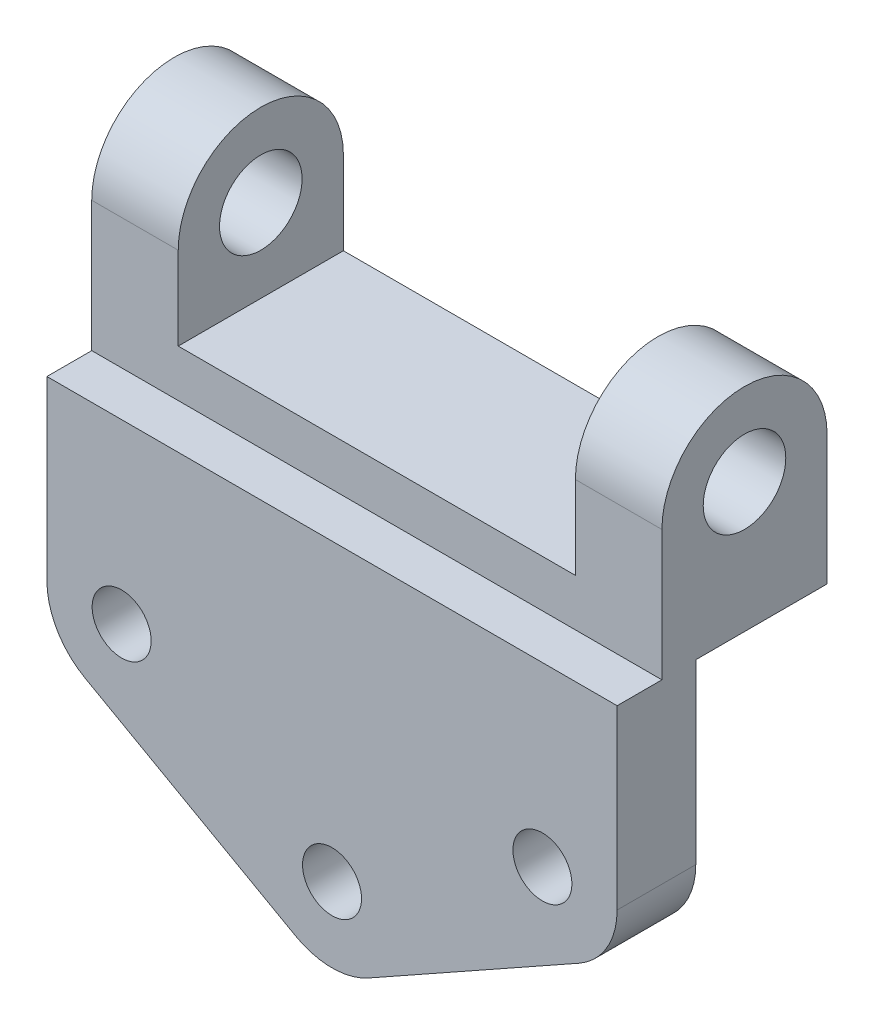
ISO-10303-21;
HEADER;
FILE_DESCRIPTION(('STEP AP214'),'2;1');
FILE_NAME('part.step','',(''),(''),'','','');
FILE_SCHEMA(('AUTOMOTIVE_DESIGN { 1 0 10303 214 1 1 1 1 }'));
ENDSEC;
DATA;
#1=APPLICATION_CONTEXT('core data for automotive mechanical design processes');
#2=APPLICATION_PROTOCOL_DEFINITION('international standard','automotive_design',2000,#1);
#3=PRODUCT_CONTEXT('',#1,'mechanical');
#4=PRODUCT('Part','Part','',(#3));
#5=PRODUCT_RELATED_PRODUCT_CATEGORY('part','',(#4));
#6=PRODUCT_DEFINITION_FORMATION('','',#4);
#7=PRODUCT_DEFINITION_CONTEXT('part definition',#1,'design');
#8=PRODUCT_DEFINITION('design','',#6,#7);
#9=PRODUCT_DEFINITION_SHAPE('','',#8);
#10=(LENGTH_UNIT() NAMED_UNIT(*) SI_UNIT(.MILLI.,.METRE.));
#11=(NAMED_UNIT(*) PLANE_ANGLE_UNIT() SI_UNIT($,.RADIAN.));
#12=(NAMED_UNIT(*) SI_UNIT($,.STERADIAN.) SOLID_ANGLE_UNIT());
#13=UNCERTAINTY_MEASURE_WITH_UNIT(LENGTH_MEASURE(1.E-05),#10,'distance_accuracy_value','');
#14=(GEOMETRIC_REPRESENTATION_CONTEXT(3) GLOBAL_UNCERTAINTY_ASSIGNED_CONTEXT((#13)) GLOBAL_UNIT_ASSIGNED_CONTEXT((#10,
#11,#12)) REPRESENTATION_CONTEXT('',''));
#15=CARTESIAN_POINT('',(0.,0.,0.));
#16=DIRECTION('',(0.,0.,1.));
#17=DIRECTION('',(1.,0.,0.));
#18=AXIS2_PLACEMENT_3D('',#15,#16,#17);
#19=CARTESIAN_POINT('',(72.5,33.,-12.3921818654785));
#20=DIRECTION('',(1.,0.,0.));
#21=DIRECTION('',(0.,0.,-1.));
#22=AXIS2_PLACEMENT_3D('',#19,#20,#21);
#23=PLANE('',#22);
#24=CARTESIAN_POINT('',(72.5,33.,-12.3921818654785));
#25=DIRECTION('',(1.,0.,0.));
#26=DIRECTION('',(0.,0.,-1.));
#27=AXIS2_PLACEMENT_3D('',#24,#25,#26);
#28=CIRCLE('',#27,10.5);
#29=CARTESIAN_POINT('',(72.5,33.,-22.8921818654785));
#30=VERTEX_POINT('',#29);
#31=EDGE_CURVE('E272',#30,#30,#28,.T.);
#32=ORIENTED_EDGE('',*,*,#31,.F.);
#33=EDGE_LOOP('',(#32));
#34=FACE_BOUND('',#33,.T.);
#35=DIRECTION('',(0.,-1.,0.));
#36=VECTOR('',#35,1.);
#37=CARTESIAN_POINT('',(72.5,-0.114515685512906,20.));
#38=LINE('',#37,#36);
#39=CARTESIAN_POINT('',(72.5,-0.114515685512906,20.));
#40=VERTEX_POINT('',#39);
#41=CARTESIAN_POINT('',(72.5,-45.1145156855129,20.));
#42=VERTEX_POINT('',#41);
#43=EDGE_CURVE('E288',#40,#42,#38,.T.);
#44=ORIENTED_EDGE('',*,*,#43,.T.);
#45=DIRECTION('',(0.,0.,1.));
#46=VECTOR('',#45,1.);
#47=CARTESIAN_POINT('',(72.5,-45.1145156855129,-125.));
#48=LINE('',#47,#46);
#49=CARTESIAN_POINT('',(72.5,-45.1145156855129,0.));
#50=VERTEX_POINT('',#49);
#51=EDGE_CURVE('E243',#50,#42,#48,.T.);
#52=ORIENTED_EDGE('',*,*,#51,.F.);
#53=DIRECTION('',(0.,1.,0.));
#54=VECTOR('',#53,1.);
#55=CARTESIAN_POINT('',(72.5,-75.1145156855129,0.));
#56=LINE('',#55,#54);
#57=CARTESIAN_POINT('',(72.5,0.,0.));
#58=VERTEX_POINT('',#57);
#59=EDGE_CURVE('E292',#50,#58,#56,.T.);
#60=ORIENTED_EDGE('',*,*,#59,.T.);
#61=DIRECTION('',(0.,0.,-1.));
#62=VECTOR('',#61,1.);
#63=CARTESIAN_POINT('',(72.5,0.,0.));
#64=LINE('',#63,#62);
#65=CARTESIAN_POINT('',(72.5,0.,-33.3921818654785));
#66=VERTEX_POINT('',#65);
#67=EDGE_CURVE('E291',#58,#66,#64,.T.);
#68=ORIENTED_EDGE('',*,*,#67,.T.);
#69=DIRECTION('',(0.,1.,0.));
#70=VECTOR('',#69,1.);
#71=CARTESIAN_POINT('',(72.5,0.,-33.3921818654785));
#72=LINE('',#71,#70);
#73=CARTESIAN_POINT('',(72.5,33.,-33.3921818654785));
#74=VERTEX_POINT('',#73);
#75=EDGE_CURVE('E293',#66,#74,#72,.T.);
#76=ORIENTED_EDGE('',*,*,#75,.T.);
#77=CARTESIAN_POINT('',(72.5,33.,-12.3921818654785));
#78=DIRECTION('',(1.,0.,0.));
#79=DIRECTION('',(0.,0.,-1.));
#80=AXIS2_PLACEMENT_3D('',#77,#78,#79);
#81=CIRCLE('',#80,21.);
#82=CARTESIAN_POINT('',(72.5,33.,8.60781813452149));
#83=VERTEX_POINT('',#82);
#84=EDGE_CURVE('E278',#74,#83,#81,.T.);
#85=ORIENTED_EDGE('',*,*,#84,.T.);
#86=DIRECTION('',(0.,-1.,0.));
#87=VECTOR('',#86,1.);
#88=CARTESIAN_POINT('',(72.5,33.,8.60781813452149));
#89=LINE('',#88,#87);
#90=CARTESIAN_POINT('',(72.5,-0.114515685512906,8.60781813452149));
#91=VERTEX_POINT('',#90);
#92=EDGE_CURVE('E282',#83,#91,#89,.T.);
#93=ORIENTED_EDGE('',*,*,#92,.T.);
#94=DIRECTION('',(0.,0.,1.));
#95=VECTOR('',#94,1.);
#96=CARTESIAN_POINT('',(72.5,-0.114515685512906,8.60781813452149));
#97=LINE('',#96,#95);
#98=EDGE_CURVE('E286',#91,#40,#97,.T.);
#99=ORIENTED_EDGE('',*,*,#98,.T.);
#100=EDGE_LOOP('',(#44,#52,#60,#68,#76,#85,#93,#99));
#101=FACE_BOUND('',#100,.T.);
#102=ADVANCED_FACE('F82',(#34,#101),#23,.T.);
#103=CARTESIAN_POINT('',(72.5,33.,-12.3921818654785));
#104=DIRECTION('',(-1.,0.,0.));
#105=DIRECTION('',(0.,0.,1.));
#106=AXIS2_PLACEMENT_3D('',#103,#104,#105);
#107=CYLINDRICAL_SURFACE('',#106,21.);
#108=CARTESIAN_POINT('',(50.5,33.,-12.3921818654785));
#109=DIRECTION('',(-1.,0.,0.));
#110=DIRECTION('',(0.,0.,1.));
#111=AXIS2_PLACEMENT_3D('',#108,#109,#110);
#112=CIRCLE('',#111,21.);
#113=CARTESIAN_POINT('',(50.5,33.,8.60781813452149));
#114=VERTEX_POINT('',#113);
#115=CARTESIAN_POINT('',(50.5,33.,-33.3921818654785));
#116=VERTEX_POINT('',#115);
#117=EDGE_CURVE('E264',#114,#116,#112,.T.);
#118=ORIENTED_EDGE('',*,*,#117,.F.);
#119=DIRECTION('',(-1.,0.,0.));
#120=VECTOR('',#119,1.);
#121=CARTESIAN_POINT('',(72.5,33.,8.60781813452149));
#122=LINE('',#121,#120);
#123=EDGE_CURVE('E327',#83,#114,#122,.T.);
#124=ORIENTED_EDGE('',*,*,#123,.F.);
#125=ORIENTED_EDGE('',*,*,#84,.F.);
#126=DIRECTION('',(-1.,0.,0.));
#127=VECTOR('',#126,1.);
#128=CARTESIAN_POINT('',(72.5,33.,-33.3921818654785));
#129=LINE('',#128,#127);
#130=EDGE_CURVE('E315',#74,#116,#129,.T.);
#131=ORIENTED_EDGE('',*,*,#130,.T.);
#132=EDGE_LOOP('',(#118,#124,#125,#131));
#133=FACE_BOUND('',#132,.T.);
#134=ADVANCED_FACE('F387',(#133),#107,.T.);
#135=CARTESIAN_POINT('',(72.5,33.,8.60781813452149));
#136=DIRECTION('',(0.,0.,-1.));
#137=DIRECTION('',(-1.,0.,0.));
#138=AXIS2_PLACEMENT_3D('',#135,#136,#137);
#139=PLANE('',#138);
#140=DIRECTION('',(0.,1.,0.));
#141=VECTOR('',#140,1.);
#142=CARTESIAN_POINT('',(50.5,33.,8.60781813452149));
#143=LINE('',#142,#141);
#144=CARTESIAN_POINT('',(50.5,11.8854843144871,8.60781813452149));
#145=VERTEX_POINT('',#144);
#146=EDGE_CURVE('E270',#145,#114,#143,.T.);
#147=ORIENTED_EDGE('',*,*,#146,.F.);
#148=DIRECTION('',(-1.,0.,0.));
#149=VECTOR('',#148,1.);
#150=CARTESIAN_POINT('',(72.5,11.8854843144871,8.60781813452149));
#151=LINE('',#150,#149);
#152=CARTESIAN_POINT('',(-50.5,11.8854843144871,8.60781813452149));
#153=VERTEX_POINT('',#152);
#154=EDGE_CURVE('E267',#145,#153,#151,.T.);
#155=ORIENTED_EDGE('',*,*,#154,.T.);
#156=DIRECTION('',(0.,1.,0.));
#157=VECTOR('',#156,1.);
#158=CARTESIAN_POINT('',(-50.5,33.,8.60781813452149));
#159=LINE('',#158,#157);
#160=CARTESIAN_POINT('',(-50.5,33.,8.60781813452149));
#161=VERTEX_POINT('',#160);
#162=EDGE_CURVE('E259',#153,#161,#159,.T.);
#163=ORIENTED_EDGE('',*,*,#162,.T.);
#164=CARTESIAN_POINT('',(-72.5,33.,8.60781813452149));
#165=VERTEX_POINT('',#164);
#166=EDGE_CURVE('E330',#161,#165,#122,.T.);
#167=ORIENTED_EDGE('',*,*,#166,.T.);
#168=DIRECTION('',(0.,-1.,0.));
#169=VECTOR('',#168,1.);
#170=CARTESIAN_POINT('',(-72.5,33.,8.60781813452149));
#171=LINE('',#170,#169);
#172=CARTESIAN_POINT('',(-72.5,-0.114515685512906,8.60781813452149));
#173=VERTEX_POINT('',#172);
#174=EDGE_CURVE('E296',#165,#173,#171,.T.);
#175=ORIENTED_EDGE('',*,*,#174,.T.);
#176=DIRECTION('',(-1.,0.,0.));
#177=VECTOR('',#176,1.);
#178=CARTESIAN_POINT('',(72.5,-0.114515685512906,8.60781813452149));
#179=LINE('',#178,#177);
#180=EDGE_CURVE('E322',#91,#173,#179,.T.);
#181=ORIENTED_EDGE('',*,*,#180,.F.);
#182=ORIENTED_EDGE('',*,*,#92,.F.);
#183=ORIENTED_EDGE('',*,*,#123,.T.);
#184=EDGE_LOOP('',(#147,#155,#163,#167,#175,#181,#182,#183));
#185=FACE_BOUND('',#184,.T.);
#186=ADVANCED_FACE('F386',(#185),#139,.F.);
#187=CARTESIAN_POINT('',(72.5,-0.114515685512906,20.));
#188=DIRECTION('',(0.,0.,-1.));
#189=DIRECTION('',(0.,1.,0.));
#190=AXIS2_PLACEMENT_3D('',#187,#188,#189);
#191=PLANE('',#190);
#192=DIRECTION('',(0.872227864306251,-0.489099736994159,0.));
#193=VECTOR('',#192,1.);
#194=CARTESIAN_POINT('',(-41.3372295567459,-73.718059376197,20.));
#195=LINE('',#194,#193);
#196=CARTESIAN_POINT('',(-62.792895002889,-61.6868451073317,20.));
#197=VERTEX_POINT('',#196);
#198=CARTESIAN_POINT('',(-9.29289500288903,-91.6868451073317,20.));
#199=VERTEX_POINT('',#198);
#200=EDGE_CURVE('E197',#197,#199,#195,.T.);
#201=ORIENTED_EDGE('',*,*,#200,.T.);
#202=CARTESIAN_POINT('',(0.,-75.1145156855129,20.));
#203=DIRECTION('',(0.,0.,1.));
#204=DIRECTION('',(1.,0.,0.));
#205=AXIS2_PLACEMENT_3D('',#202,#203,#204);
#206=CIRCLE('',#205,19.);
#207=CARTESIAN_POINT('',(9.29289500288903,-91.6868451073317,20.));
#208=VERTEX_POINT('',#207);
#209=EDGE_CURVE('E201',#199,#208,#206,.T.);
#210=ORIENTED_EDGE('',*,*,#209,.T.);
#211=DIRECTION('',(-0.872227864306251,-0.489099736994159,0.));
#212=VECTOR('',#211,1.);
#213=CARTESIAN_POINT('',(41.3372295567459,-73.718059376197,20.));
#214=LINE('',#213,#212);
#215=CARTESIAN_POINT('',(62.792895002889,-61.6868451073317,20.));
#216=VERTEX_POINT('',#215);
#217=EDGE_CURVE('E242',#216,#208,#214,.T.);
#218=ORIENTED_EDGE('',*,*,#217,.F.);
#219=CARTESIAN_POINT('',(53.5,-45.1145156855129,20.));
#220=DIRECTION('',(0.,0.,1.));
#221=DIRECTION('',(1.,0.,0.));
#222=AXIS2_PLACEMENT_3D('',#219,#220,#221);
#223=CIRCLE('',#222,19.);
#224=EDGE_CURVE('E246',#42,#216,#223,.F.);
#225=ORIENTED_EDGE('',*,*,#224,.F.);
#226=ORIENTED_EDGE('',*,*,#43,.F.);
#227=DIRECTION('',(-1.,0.,0.));
#228=VECTOR('',#227,1.);
#229=CARTESIAN_POINT('',(72.5,-0.114515685512906,20.));
#230=LINE('',#229,#228);
#231=CARTESIAN_POINT('',(-72.5,-0.114515685512906,20.));
#232=VERTEX_POINT('',#231);
#233=EDGE_CURVE('E321',#40,#232,#230,.T.);
#234=ORIENTED_EDGE('',*,*,#233,.T.);
#235=DIRECTION('',(0.,-1.,0.));
#236=VECTOR('',#235,1.);
#237=CARTESIAN_POINT('',(-72.5,-0.114515685512906,20.));
#238=LINE('',#237,#236);
#239=CARTESIAN_POINT('',(-72.5,-45.1145156855129,20.));
#240=VERTEX_POINT('',#239);
#241=EDGE_CURVE('E302',#232,#240,#238,.T.);
#242=ORIENTED_EDGE('',*,*,#241,.T.);
#243=CARTESIAN_POINT('',(-53.5,-45.1145156855129,20.));
#244=DIRECTION('',(0.,0.,1.));
#245=DIRECTION('',(1.,0.,0.));
#246=AXIS2_PLACEMENT_3D('',#243,#244,#245);
#247=CIRCLE('',#246,19.);
#248=EDGE_CURVE('E202',#240,#197,#247,.T.);
#249=ORIENTED_EDGE('',*,*,#248,.T.);
#250=EDGE_LOOP('',(#201,#210,#218,#225,#226,#234,#242,#249));
#251=FACE_BOUND('',#250,.T.);
#252=CARTESIAN_POINT('',(-53.5,-45.1145156855129,20.));
#253=DIRECTION('',(0.,0.,1.));
#254=DIRECTION('',(1.,0.,0.));
#255=AXIS2_PLACEMENT_3D('',#252,#253,#254);
#256=CIRCLE('',#255,7.5);
#257=CARTESIAN_POINT('',(-46.,-45.1145156855129,20.));
#258=VERTEX_POINT('',#257);
#259=EDGE_CURVE('E230',#258,#258,#256,.T.);
#260=ORIENTED_EDGE('',*,*,#259,.F.);
#261=EDGE_LOOP('',(#260));
#262=FACE_BOUND('',#261,.T.);
#263=CARTESIAN_POINT('',(0.,-75.1145156855129,20.));
#264=DIRECTION('',(0.,0.,1.));
#265=DIRECTION('',(1.,0.,0.));
#266=AXIS2_PLACEMENT_3D('',#263,#264,#265);
#267=CIRCLE('',#266,7.5);
#268=CARTESIAN_POINT('',(7.5,-75.1145156855129,20.));
#269=VERTEX_POINT('',#268);
#270=EDGE_CURVE('E228',#269,#269,#267,.T.);
#271=ORIENTED_EDGE('',*,*,#270,.F.);
#272=EDGE_LOOP('',(#271));
#273=FACE_BOUND('',#272,.T.);
#274=CARTESIAN_POINT('',(53.5,-45.1145156855129,20.));
#275=DIRECTION('',(0.,0.,1.));
#276=DIRECTION('',(1.,0.,0.));
#277=AXIS2_PLACEMENT_3D('',#274,#275,#276);
#278=CIRCLE('',#277,7.5);
#279=CARTESIAN_POINT('',(61.,-45.1145156855129,20.));
#280=VERTEX_POINT('',#279);
#281=EDGE_CURVE('E233',#280,#280,#278,.F.);
#282=ORIENTED_EDGE('',*,*,#281,.T.);
#283=EDGE_LOOP('',(#282));
#284=FACE_BOUND('',#283,.T.);
#285=ADVANCED_FACE('F200',(#251,#262,#273,#284),#191,.F.);
#286=CARTESIAN_POINT('',(72.5,-75.1145156855129,0.));
#287=DIRECTION('',(0.,0.,1.));
#288=DIRECTION('',(1.,0.,0.));
#289=AXIS2_PLACEMENT_3D('',#286,#287,#288);
#290=PLANE('',#289);
#291=CARTESIAN_POINT('',(0.,-75.1145156855129,0.));
#292=DIRECTION('',(0.,0.,1.));
#293=DIRECTION('',(1.,0.,0.));
#294=AXIS2_PLACEMENT_3D('',#291,#292,#293);
#295=CIRCLE('',#294,19.);
#296=CARTESIAN_POINT('',(9.29289500288902,-91.6868451073317,0.));
#297=VERTEX_POINT('',#296);
#298=CARTESIAN_POINT('',(-9.29289500288903,-91.6868451073317,0.));
#299=VERTEX_POINT('',#298);
#300=EDGE_CURVE('E221',#297,#299,#295,.F.);
#301=ORIENTED_EDGE('',*,*,#300,.T.);
#302=DIRECTION('',(0.872227864306251,-0.489099736994159,0.));
#303=VECTOR('',#302,1.);
#304=CARTESIAN_POINT('',(45.8637599243487,-122.615810487091,0.));
#305=LINE('',#304,#303);
#306=CARTESIAN_POINT('',(-62.792895002889,-61.6868451073317,0.));
#307=VERTEX_POINT('',#306);
#308=EDGE_CURVE('E215',#307,#299,#305,.T.);
#309=ORIENTED_EDGE('',*,*,#308,.F.);
#310=CARTESIAN_POINT('',(-53.5,-45.1145156855129,0.));
#311=DIRECTION('',(0.,0.,1.));
#312=DIRECTION('',(1.,0.,0.));
#313=AXIS2_PLACEMENT_3D('',#310,#311,#312);
#314=CIRCLE('',#313,19.);
#315=CARTESIAN_POINT('',(-72.5,-45.1145156855129,0.));
#316=VERTEX_POINT('',#315);
#317=EDGE_CURVE('E340',#316,#307,#314,.T.);
#318=ORIENTED_EDGE('',*,*,#317,.F.);
#319=DIRECTION('',(0.,1.,0.));
#320=VECTOR('',#319,1.);
#321=CARTESIAN_POINT('',(-72.5,-75.1145156855129,0.));
#322=LINE('',#321,#320);
#323=CARTESIAN_POINT('',(-72.5,0.,0.));
#324=VERTEX_POINT('',#323);
#325=EDGE_CURVE('E308',#316,#324,#322,.T.);
#326=ORIENTED_EDGE('',*,*,#325,.T.);
#327=DIRECTION('',(-1.,0.,0.));
#328=VECTOR('',#327,1.);
#329=CARTESIAN_POINT('',(72.5,0.,0.));
#330=LINE('',#329,#328);
#331=EDGE_CURVE('E318',#58,#324,#330,.T.);
#332=ORIENTED_EDGE('',*,*,#331,.F.);
#333=ORIENTED_EDGE('',*,*,#59,.F.);
#334=CARTESIAN_POINT('',(53.5,-45.1145156855129,0.));
#335=DIRECTION('',(0.,0.,1.));
#336=DIRECTION('',(1.,0.,0.));
#337=AXIS2_PLACEMENT_3D('',#334,#335,#336);
#338=CIRCLE('',#337,19.);
#339=CARTESIAN_POINT('',(62.792895002889,-61.6868451073317,0.));
#340=VERTEX_POINT('',#339);
#341=EDGE_CURVE('E91',#50,#340,#338,.F.);
#342=ORIENTED_EDGE('',*,*,#341,.T.);
#343=DIRECTION('',(-0.872227864306251,-0.489099736994159,0.));
#344=VECTOR('',#343,1.);
#345=CARTESIAN_POINT('',(64.4495499301267,-60.7578797275722,0.));
#346=LINE('',#345,#344);
#347=EDGE_CURVE('E12',#340,#297,#346,.T.);
#348=ORIENTED_EDGE('',*,*,#347,.T.);
#349=EDGE_LOOP('',(#301,#309,#318,#326,#332,#333,#342,#348));
#350=FACE_BOUND('',#349,.T.);
#351=CARTESIAN_POINT('',(-53.5,-45.1145156855129,0.));
#352=DIRECTION('',(0.,0.,1.));
#353=DIRECTION('',(1.,0.,0.));
#354=AXIS2_PLACEMENT_3D('',#351,#352,#353);
#355=CIRCLE('',#354,7.5);
#356=CARTESIAN_POINT('',(-46.,-45.1145156855129,0.));
#357=VERTEX_POINT('',#356);
#358=EDGE_CURVE('E86',#357,#357,#355,.T.);
#359=ORIENTED_EDGE('',*,*,#358,.T.);
#360=EDGE_LOOP('',(#359));
#361=FACE_BOUND('',#360,.T.);
#362=CARTESIAN_POINT('',(0.,-75.1145156855129,0.));
#363=DIRECTION('',(0.,0.,1.));
#364=DIRECTION('',(1.,0.,0.));
#365=AXIS2_PLACEMENT_3D('',#362,#363,#364);
#366=CIRCLE('',#365,7.5);
#367=CARTESIAN_POINT('',(7.5,-75.1145156855129,0.));
#368=VERTEX_POINT('',#367);
#369=EDGE_CURVE('E341',#368,#368,#366,.T.);
#370=ORIENTED_EDGE('',*,*,#369,.T.);
#371=EDGE_LOOP('',(#370));
#372=FACE_BOUND('',#371,.T.);
#373=CARTESIAN_POINT('',(53.5,-45.1145156855129,0.));
#374=DIRECTION('',(0.,0.,1.));
#375=DIRECTION('',(1.,0.,0.));
#376=AXIS2_PLACEMENT_3D('',#373,#374,#375);
#377=CIRCLE('',#376,7.5);
#378=CARTESIAN_POINT('',(61.,-45.1145156855129,0.));
#379=VERTEX_POINT('',#378);
#380=EDGE_CURVE('E275',#379,#379,#377,.F.);
#381=ORIENTED_EDGE('',*,*,#380,.F.);
#382=EDGE_LOOP('',(#381));
#383=FACE_BOUND('',#382,.T.);
#384=ADVANCED_FACE('F349',(#350,#361,#372,#383),#290,.F.);
#385=CARTESIAN_POINT('',(72.5,0.,-33.3921818654785));
#386=DIRECTION('',(0.,0.,1.));
#387=DIRECTION('',(1.,0.,0.));
#388=AXIS2_PLACEMENT_3D('',#385,#386,#387);
#389=PLANE('',#388);
#390=DIRECTION('',(0.,-1.,0.));
#391=VECTOR('',#390,1.);
#392=CARTESIAN_POINT('',(50.5,0.,-33.3921818654785));
#393=LINE('',#392,#391);
#394=CARTESIAN_POINT('',(50.5,11.8854843144871,-33.3921818654785));
#395=VERTEX_POINT('',#394);
#396=EDGE_CURVE('E263',#116,#395,#393,.T.);
#397=ORIENTED_EDGE('',*,*,#396,.F.);
#398=ORIENTED_EDGE('',*,*,#130,.F.);
#399=ORIENTED_EDGE('',*,*,#75,.F.);
#400=DIRECTION('',(-1.,0.,0.));
#401=VECTOR('',#400,1.);
#402=CARTESIAN_POINT('',(72.5,0.,-33.3921818654785));
#403=LINE('',#402,#401);
#404=CARTESIAN_POINT('',(-72.5,0.,-33.3921818654785));
#405=VERTEX_POINT('',#404);
#406=EDGE_CURVE('E312',#66,#405,#403,.T.);
#407=ORIENTED_EDGE('',*,*,#406,.T.);
#408=DIRECTION('',(0.,1.,0.));
#409=VECTOR('',#408,1.);
#410=CARTESIAN_POINT('',(-72.5,0.,-33.3921818654785));
#411=LINE('',#410,#409);
#412=CARTESIAN_POINT('',(-72.5,33.,-33.3921818654785));
#413=VERTEX_POINT('',#412);
#414=EDGE_CURVE('E285',#405,#413,#411,.T.);
#415=ORIENTED_EDGE('',*,*,#414,.T.);
#416=CARTESIAN_POINT('',(-50.5,33.,-33.3921818654785));
#417=VERTEX_POINT('',#416);
#418=EDGE_CURVE('E299',#417,#413,#129,.T.);
#419=ORIENTED_EDGE('',*,*,#418,.F.);
#420=DIRECTION('',(0.,-1.,0.));
#421=VECTOR('',#420,1.);
#422=CARTESIAN_POINT('',(-50.5,0.,-33.3921818654785));
#423=LINE('',#422,#421);
#424=CARTESIAN_POINT('',(-50.5,11.8854843144871,-33.3921818654785));
#425=VERTEX_POINT('',#424);
#426=EDGE_CURVE('E251',#417,#425,#423,.T.);
#427=ORIENTED_EDGE('',*,*,#426,.T.);
#428=DIRECTION('',(1.,0.,0.));
#429=VECTOR('',#428,1.);
#430=CARTESIAN_POINT('',(72.5,11.8854843144871,-33.3921818654785));
#431=LINE('',#430,#429);
#432=EDGE_CURVE('E332',#425,#395,#431,.T.);
#433=ORIENTED_EDGE('',*,*,#432,.T.);
#434=EDGE_LOOP('',(#397,#398,#399,#407,#415,#419,#427,#433));
#435=FACE_BOUND('',#434,.T.);
#436=ADVANCED_FACE('F378',(#435),#389,.F.);
#437=CARTESIAN_POINT('',(72.5,33.,-12.3921818654785));
#438=DIRECTION('',(-1.,0.,0.));
#439=DIRECTION('',(0.,0.,1.));
#440=AXIS2_PLACEMENT_3D('',#437,#438,#439);
#441=CYLINDRICAL_SURFACE('',#440,10.5);
#442=ORIENTED_EDGE('',*,*,#31,.T.);
#443=EDGE_LOOP('',(#442));
#444=FACE_BOUND('',#443,.T.);
#445=CARTESIAN_POINT('',(50.5,33.,-12.3921818654785));
#446=DIRECTION('',(-1.,0.,0.));
#447=DIRECTION('',(0.,0.,1.));
#448=AXIS2_PLACEMENT_3D('',#445,#446,#447);
#449=CIRCLE('',#448,10.5);
#450=CARTESIAN_POINT('',(50.5,33.,-1.89218186547851));
#451=VERTEX_POINT('',#450);
#452=EDGE_CURVE('E265',#451,#451,#449,.T.);
#453=ORIENTED_EDGE('',*,*,#452,.T.);
#454=EDGE_LOOP('',(#453));
#455=FACE_BOUND('',#454,.T.);
#456=ADVANCED_FACE('F431',(#444,#455),#441,.F.);
#457=CARTESIAN_POINT('',(-72.5,33.,-12.3921818654785));
#458=DIRECTION('',(1.,0.,0.));
#459=DIRECTION('',(0.,0.,-1.));
#460=AXIS2_PLACEMENT_3D('',#457,#458,#459);
#461=PLANE('',#460);
#462=ORIENTED_EDGE('',*,*,#325,.F.);
#463=DIRECTION('',(0.,0.,1.));
#464=VECTOR('',#463,1.);
#465=CARTESIAN_POINT('',(-72.5,-45.1145156855129,-125.));
#466=LINE('',#465,#464);
#467=EDGE_CURVE('E206',#316,#240,#466,.T.);
#468=ORIENTED_EDGE('',*,*,#467,.T.);
#469=ORIENTED_EDGE('',*,*,#241,.F.);
#470=DIRECTION('',(0.,0.,1.));
#471=VECTOR('',#470,1.);
#472=CARTESIAN_POINT('',(-72.5,-0.114515685512906,8.60781813452149));
#473=LINE('',#472,#471);
#474=EDGE_CURVE('E305',#173,#232,#473,.T.);
#475=ORIENTED_EDGE('',*,*,#474,.F.);
#476=ORIENTED_EDGE('',*,*,#174,.F.);
#477=CARTESIAN_POINT('',(-72.5,33.,-12.3921818654785));
#478=DIRECTION('',(1.,0.,0.));
#479=DIRECTION('',(0.,0.,-1.));
#480=AXIS2_PLACEMENT_3D('',#477,#478,#479);
#481=CIRCLE('',#480,21.);
#482=EDGE_CURVE('E277',#413,#165,#481,.T.);
#483=ORIENTED_EDGE('',*,*,#482,.F.);
#484=ORIENTED_EDGE('',*,*,#414,.F.);
#485=DIRECTION('',(0.,0.,-1.));
#486=VECTOR('',#485,1.);
#487=CARTESIAN_POINT('',(-72.5,0.,0.));
#488=LINE('',#487,#486);
#489=EDGE_CURVE('E306',#324,#405,#488,.T.);
#490=ORIENTED_EDGE('',*,*,#489,.F.);
#491=EDGE_LOOP('',(#462,#468,#469,#475,#476,#483,#484,#490));
#492=FACE_BOUND('',#491,.T.);
#493=CARTESIAN_POINT('',(-72.5,33.,-12.3921818654785));
#494=DIRECTION('',(1.,0.,0.));
#495=DIRECTION('',(0.,0.,-1.));
#496=AXIS2_PLACEMENT_3D('',#493,#494,#495);
#497=CIRCLE('',#496,10.5);
#498=CARTESIAN_POINT('',(-72.5,33.,-22.8921818654785));
#499=VERTEX_POINT('',#498);
#500=EDGE_CURVE('E280',#499,#499,#497,.T.);
#501=ORIENTED_EDGE('',*,*,#500,.T.);
#502=EDGE_LOOP('',(#501));
#503=FACE_BOUND('',#502,.T.);
#504=ADVANCED_FACE('F370',(#492,#503),#461,.F.);
#505=ORIENTED_EDGE('',*,*,#166,.F.);
#506=CARTESIAN_POINT('',(-50.5,33.,-12.3921818654785));
#507=DIRECTION('',(-1.,0.,0.));
#508=DIRECTION('',(0.,-1.,0.));
#509=AXIS2_PLACEMENT_3D('',#506,#507,#508);
#510=CIRCLE('',#509,21.);
#511=EDGE_CURVE('E258',#161,#417,#510,.T.);
#512=ORIENTED_EDGE('',*,*,#511,.T.);
#513=ORIENTED_EDGE('',*,*,#418,.T.);
#514=ORIENTED_EDGE('',*,*,#482,.T.);
#515=EDGE_LOOP('',(#505,#512,#513,#514));
#516=FACE_BOUND('',#515,.T.);
#517=ADVANCED_FACE('F88',(#516),#107,.T.);
#518=CARTESIAN_POINT('',(72.5,-0.114515685512906,8.60781813452149));
#519=DIRECTION('',(0.,-1.,0.));
#520=DIRECTION('',(0.,0.,-1.));
#521=AXIS2_PLACEMENT_3D('',#518,#519,#520);
#522=PLANE('',#521);
#523=ORIENTED_EDGE('',*,*,#474,.T.);
#524=ORIENTED_EDGE('',*,*,#233,.F.);
#525=ORIENTED_EDGE('',*,*,#98,.F.);
#526=ORIENTED_EDGE('',*,*,#180,.T.);
#527=EDGE_LOOP('',(#523,#524,#525,#526));
#528=FACE_BOUND('',#527,.T.);
#529=ADVANCED_FACE('F392',(#528),#522,.F.);
#530=CARTESIAN_POINT('',(72.5,0.,0.));
#531=DIRECTION('',(0.,1.,0.));
#532=DIRECTION('',(0.,0.,1.));
#533=AXIS2_PLACEMENT_3D('',#530,#531,#532);
#534=PLANE('',#533);
#535=ORIENTED_EDGE('',*,*,#489,.T.);
#536=ORIENTED_EDGE('',*,*,#406,.F.);
#537=ORIENTED_EDGE('',*,*,#67,.F.);
#538=ORIENTED_EDGE('',*,*,#331,.T.);
#539=EDGE_LOOP('',(#535,#536,#537,#538));
#540=FACE_BOUND('',#539,.T.);
#541=ADVANCED_FACE('F373',(#540),#534,.F.);
#542=CARTESIAN_POINT('',(-50.5,33.,-12.3921818654785));
#543=DIRECTION('',(-1.,0.,0.));
#544=DIRECTION('',(0.,-1.,0.));
#545=AXIS2_PLACEMENT_3D('',#542,#543,#544);
#546=CIRCLE('',#545,10.5);
#547=CARTESIAN_POINT('',(-50.5,22.5,-12.3921818654785));
#548=VERTEX_POINT('',#547);
#549=EDGE_CURVE('E249',#548,#548,#546,.T.);
#550=ORIENTED_EDGE('',*,*,#549,.F.);
#551=EDGE_LOOP('',(#550));
#552=FACE_BOUND('',#551,.T.);
#553=ORIENTED_EDGE('',*,*,#500,.F.);
#554=EDGE_LOOP('',(#553));
#555=FACE_BOUND('',#554,.T.);
#556=ADVANCED_FACE('F412',(#552,#555),#441,.F.);
#557=CARTESIAN_POINT('',(0.,11.8854843144871,-125.));
#558=DIRECTION('',(0.,-1.,0.));
#559=DIRECTION('',(1.,0.,0.));
#560=AXIS2_PLACEMENT_3D('',#557,#558,#559);
#561=PLANE('',#560);
#562=DIRECTION('',(0.,0.,1.));
#563=VECTOR('',#562,1.);
#564=CARTESIAN_POINT('',(50.5,11.8854843144871,-125.));
#565=LINE('',#564,#563);
#566=EDGE_CURVE('E232',#395,#145,#565,.T.);
#567=ORIENTED_EDGE('',*,*,#566,.F.);
#568=ORIENTED_EDGE('',*,*,#432,.F.);
#569=DIRECTION('',(0.,0.,1.));
#570=VECTOR('',#569,1.);
#571=CARTESIAN_POINT('',(-50.5,11.8854843144871,-125.));
#572=LINE('',#571,#570);
#573=EDGE_CURVE('E226',#425,#153,#572,.T.);
#574=ORIENTED_EDGE('',*,*,#573,.T.);
#575=ORIENTED_EDGE('',*,*,#154,.F.);
#576=EDGE_LOOP('',(#567,#568,#574,#575));
#577=FACE_BOUND('',#576,.T.);
#578=ADVANCED_FACE('F402',(#577),#561,.F.);
#579=CARTESIAN_POINT('',(50.5,0.,-125.));
#580=DIRECTION('',(-1.,0.,0.));
#581=DIRECTION('',(0.,0.,1.));
#582=AXIS2_PLACEMENT_3D('',#579,#580,#581);
#583=PLANE('',#582);
#584=ORIENTED_EDGE('',*,*,#452,.F.);
#585=EDGE_LOOP('',(#584));
#586=FACE_BOUND('',#585,.T.);
#587=ORIENTED_EDGE('',*,*,#146,.T.);
#588=ORIENTED_EDGE('',*,*,#117,.T.);
#589=ORIENTED_EDGE('',*,*,#396,.T.);
#590=ORIENTED_EDGE('',*,*,#566,.T.);
#591=EDGE_LOOP('',(#587,#588,#589,#590));
#592=FACE_BOUND('',#591,.T.);
#593=ADVANCED_FACE('F401',(#586,#592),#583,.T.);
#594=CARTESIAN_POINT('',(-50.5,0.,-125.));
#595=DIRECTION('',(-1.,0.,0.));
#596=DIRECTION('',(0.,-1.,0.));
#597=AXIS2_PLACEMENT_3D('',#594,#595,#596);
#598=PLANE('',#597);
#599=ORIENTED_EDGE('',*,*,#549,.T.);
#600=EDGE_LOOP('',(#599));
#601=FACE_BOUND('',#600,.T.);
#602=ORIENTED_EDGE('',*,*,#573,.F.);
#603=ORIENTED_EDGE('',*,*,#426,.F.);
#604=ORIENTED_EDGE('',*,*,#511,.F.);
#605=ORIENTED_EDGE('',*,*,#162,.F.);
#606=EDGE_LOOP('',(#602,#603,#604,#605));
#607=FACE_BOUND('',#606,.T.);
#608=ADVANCED_FACE('F398',(#601,#607),#598,.F.);
#609=CARTESIAN_POINT('',(-53.5,-45.1145156855129,-125.));
#610=DIRECTION('',(0.,0.,1.));
#611=DIRECTION('',(1.,0.,0.));
#612=AXIS2_PLACEMENT_3D('',#609,#610,#611);
#613=CYLINDRICAL_SURFACE('',#612,19.);
#614=ORIENTED_EDGE('',*,*,#317,.T.);
#615=DIRECTION('',(0.,0.,1.));
#616=VECTOR('',#615,1.);
#617=CARTESIAN_POINT('',(-62.792895002889,-61.6868451073317,-125.));
#618=LINE('',#617,#616);
#619=EDGE_CURVE('E107',#307,#197,#618,.T.);
#620=ORIENTED_EDGE('',*,*,#619,.T.);
#621=ORIENTED_EDGE('',*,*,#248,.F.);
#622=ORIENTED_EDGE('',*,*,#467,.F.);
#623=EDGE_LOOP('',(#614,#620,#621,#622));
#624=FACE_BOUND('',#623,.T.);
#625=ADVANCED_FACE('F411',(#624),#613,.T.);
#626=CARTESIAN_POINT('',(-41.3372295567459,-73.718059376197,-125.));
#627=DIRECTION('',(-0.489099736994159,-0.872227864306251,0.));
#628=DIRECTION('',(0.872227864306251,-0.489099736994159,0.));
#629=AXIS2_PLACEMENT_3D('',#626,#627,#628);
#630=PLANE('',#629);
#631=ORIENTED_EDGE('',*,*,#308,.T.);
#632=DIRECTION('',(0.,0.,1.));
#633=VECTOR('',#632,1.);
#634=CARTESIAN_POINT('',(-9.29289500288903,-91.6868451073317,-79.9832551920158));
#635=LINE('',#634,#633);
#636=EDGE_CURVE('E207',#299,#199,#635,.T.);
#637=ORIENTED_EDGE('',*,*,#636,.T.);
#638=ORIENTED_EDGE('',*,*,#200,.F.);
#639=ORIENTED_EDGE('',*,*,#619,.F.);
#640=EDGE_LOOP('',(#631,#637,#638,#639));
#641=FACE_BOUND('',#640,.T.);
#642=ADVANCED_FACE('F209',(#641),#630,.T.);
#643=CARTESIAN_POINT('',(0.,-75.1145156855129,-125.));
#644=DIRECTION('',(0.,0.,1.));
#645=DIRECTION('',(1.,0.,0.));
#646=AXIS2_PLACEMENT_3D('',#643,#644,#645);
#647=CYLINDRICAL_SURFACE('',#646,7.5);
#648=ORIENTED_EDGE('',*,*,#270,.T.);
#649=EDGE_LOOP('',(#648));
#650=FACE_BOUND('',#649,.T.);
#651=ORIENTED_EDGE('',*,*,#369,.F.);
#652=EDGE_LOOP('',(#651));
#653=FACE_BOUND('',#652,.T.);
#654=ADVANCED_FACE('F513',(#650,#653),#647,.F.);
#655=CARTESIAN_POINT('',(53.5,-45.1145156855129,-125.));
#656=DIRECTION('',(0.,0.,1.));
#657=DIRECTION('',(1.,0.,0.));
#658=AXIS2_PLACEMENT_3D('',#655,#656,#657);
#659=CYLINDRICAL_SURFACE('',#658,7.5);
#660=ORIENTED_EDGE('',*,*,#281,.F.);
#661=EDGE_LOOP('',(#660));
#662=FACE_BOUND('',#661,.T.);
#663=ORIENTED_EDGE('',*,*,#380,.T.);
#664=EDGE_LOOP('',(#663));
#665=FACE_BOUND('',#664,.T.);
#666=ADVANCED_FACE('F527',(#662,#665),#659,.F.);
#667=CARTESIAN_POINT('',(41.3372295567459,-73.718059376197,-125.));
#668=DIRECTION('',(-0.489099736994159,0.872227864306251,0.));
#669=DIRECTION('',(-0.872227864306251,-0.489099736994159,0.));
#670=AXIS2_PLACEMENT_3D('',#667,#668,#669);
#671=PLANE('',#670);
#672=DIRECTION('',(0.,0.,1.));
#673=VECTOR('',#672,1.);
#674=CARTESIAN_POINT('',(62.792895002889,-61.6868451073317,-125.));
#675=LINE('',#674,#673);
#676=EDGE_CURVE('E99',#340,#216,#675,.T.);
#677=ORIENTED_EDGE('',*,*,#676,.T.);
#678=ORIENTED_EDGE('',*,*,#217,.T.);
#679=DIRECTION('',(0.,0.,1.));
#680=VECTOR('',#679,1.);
#681=CARTESIAN_POINT('',(9.29289500288903,-91.6868451073317,-79.9832551920158));
#682=LINE('',#681,#680);
#683=EDGE_CURVE('E216',#297,#208,#682,.T.);
#684=ORIENTED_EDGE('',*,*,#683,.F.);
#685=ORIENTED_EDGE('',*,*,#347,.F.);
#686=EDGE_LOOP('',(#677,#678,#684,#685));
#687=FACE_BOUND('',#686,.T.);
#688=ADVANCED_FACE('F363',(#687),#671,.F.);
#689=CARTESIAN_POINT('',(53.5,-45.1145156855129,-125.));
#690=DIRECTION('',(0.,0.,1.));
#691=DIRECTION('',(1.,0.,0.));
#692=AXIS2_PLACEMENT_3D('',#689,#690,#691);
#693=CYLINDRICAL_SURFACE('',#692,19.);
#694=ORIENTED_EDGE('',*,*,#51,.T.);
#695=ORIENTED_EDGE('',*,*,#224,.T.);
#696=ORIENTED_EDGE('',*,*,#676,.F.);
#697=ORIENTED_EDGE('',*,*,#341,.F.);
#698=EDGE_LOOP('',(#694,#695,#696,#697));
#699=FACE_BOUND('',#698,.T.);
#700=ADVANCED_FACE('F352',(#699),#693,.T.);
#701=CARTESIAN_POINT('',(-53.5,-45.1145156855129,-125.));
#702=DIRECTION('',(0.,0.,1.));
#703=DIRECTION('',(1.,0.,0.));
#704=AXIS2_PLACEMENT_3D('',#701,#702,#703);
#705=CYLINDRICAL_SURFACE('',#704,7.5);
#706=ORIENTED_EDGE('',*,*,#259,.T.);
#707=EDGE_LOOP('',(#706));
#708=FACE_BOUND('',#707,.T.);
#709=ORIENTED_EDGE('',*,*,#358,.F.);
#710=EDGE_LOOP('',(#709));
#711=FACE_BOUND('',#710,.T.);
#712=ADVANCED_FACE('F560',(#708,#711),#705,.F.);
#713=CARTESIAN_POINT('',(0.,-75.1145156855129,-79.9832551920158));
#714=DIRECTION('',(0.,0.,1.));
#715=DIRECTION('',(1.,0.,0.));
#716=AXIS2_PLACEMENT_3D('',#713,#714,#715);
#717=CYLINDRICAL_SURFACE('',#716,19.);
#718=ORIENTED_EDGE('',*,*,#300,.F.);
#719=ORIENTED_EDGE('',*,*,#683,.T.);
#720=ORIENTED_EDGE('',*,*,#209,.F.);
#721=ORIENTED_EDGE('',*,*,#636,.F.);
#722=EDGE_LOOP('',(#718,#719,#720,#721));
#723=FACE_BOUND('',#722,.T.);
#724=ADVANCED_FACE('F218',(#723),#717,.T.);
#725=CLOSED_SHELL('',(#102,#134,#186,#285,#384,#436,#456,#504,#517,#529,#541,#556,#578,#593,
#608,#625,#642,#654,#666,#688,#700,#712,#724));
#726=MANIFOLD_SOLID_BREP('B2',#725);
#727=ADVANCED_BREP_SHAPE_REPRESENTATION('',(#18,#726),#14);
#728=SHAPE_DEFINITION_REPRESENTATION(#9,#727);
ENDSEC;
END-ISO-10303-21;
